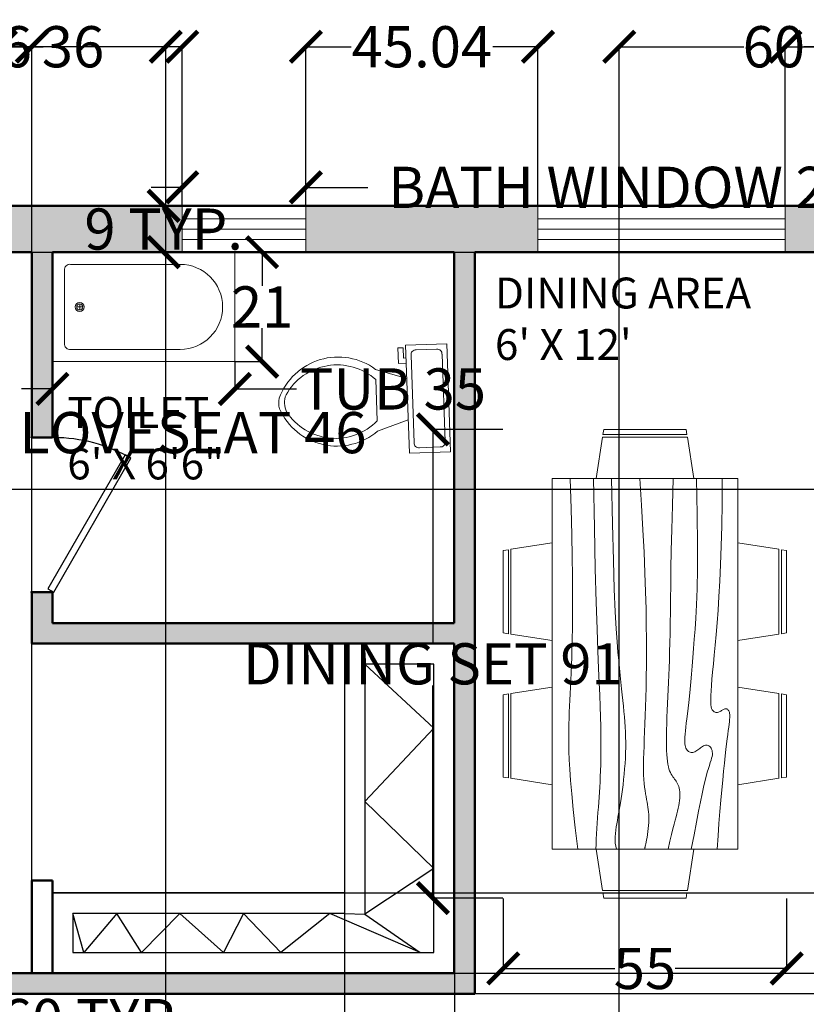
# Model space of a CAD drawing. Units: inches. Extents: x -30 to 744, y -375 to 57.
# Tile 5 of 8: x 202 to 355, y -134 to 57. Entities that reach past the tile are written whole.
import ezdxf

# ---------------------------------------------------------------- set-up
doc = ezdxf.new("R2010")
doc.units = ezdxf.units.IN
doc.header["$MEASUREMENT"] = 0
for name, color, linetype, lineweight in [('A-ANNO-DIMS', 2, 'Continuous', 18), ('A-AREA-IDEN', 7, 'Continuous', 25), ('A-DOOR', 3, 'Continuous', 25), ('A-FLOR-CASE', 8, 'Continuous', 25), ('A-FLOR-FIXT', 9, 'Continuous', 20), ('A-FURN', 8, 'Continuous', 18), ('A-GLAZ', 4, 'Continuous', 18), ('A-WALL', 7, 'Continuous', 50)]:
    doc.layers.add(name, color=color, linetype=linetype, lineweight=lineweight)
doc.layers.add('A-WALL-PATT', color=251, linetype='Continuous', lineweight=13, true_color=0x636466)
doc.styles.get("Standard").update_dxf_attribs({"font": 'arial.ttf'})
doc.dimstyles.get("Standard").update_dxf_attribs({"dimtxt": 8, "dimasz": 6, "dimexe": 0.18, "dimexo": 0.0625, "dimgap": 0.09, "dimtad": 0, "dimtih": 1, "dimtoh": 1, "dimdec": 0, "dimzin": 0, "dimdsep": 46, "dimlunit": 4, "dimtxsty": 'Standard', "dimblk": 'ARCHTICK', "dimcen": 0.09, "dimadec": 0, "dimazin": 0, "dimtfac": 1, "dimtdec": 0, "dimtofl": 0, "dimtmove": 0, "dimatfit": 1, "dimldrblk": 'ARCHTICK', "dimfxl": 1, "dimtolj": 1, "dimtzin": 0, "dimarcsym": 0})

# ---------------------------------------------------------------- blocks, each defined once
blk = doc.blocks.new('*U4')
for p, q in [((0, 0), (0, 6)), ((40, 0), (40, 6))]:
    blk.add_line(p, q)
blk.add_lwpolyline([(0, 0), (34.64, -20), (35.52, -18.48), (0.87, 1.52)], close=True)
blk.add_arc((0, 0), 40, 330, 0)
blk = doc.blocks.new('Dining Set - 36 x 72 in.')
for p, q in [((-22, 27.5), (-22.1562, 26.50042)), ((-22, 27.5), (-6, 27.5)), ((-5.8437, 26.49966), (-6, 27.5)), ((6, 27.5), (5.8438, 26.50042)), ((6, 27.5), (22, 27.5)), ((22.1563, 26.49966), (22, 27.5)), ((-22.2343, 26.00059), (-23.4847, 17.99762)), ((-22.2304, 26), (-5.7608, 26)), ((-5.8416, 26.5), (-22.1534, 26.5)), ((-4.5152, 17.99762), (-5.7655, 25.99926)), ((5.7657, 26.00059), (4.5153, 17.99762)), ((5.7696, 26), (22.2392, 26)), ((22.1584, 26.5), (5.8466, 26.5)), ((23.4848, 17.99762), (22.2345, 25.99926)), ((36, 18), (-36, 18)), ((-36, 18), (-36, -18)), ((36, -18), (36, 18)), ((-45.5, 8), (-44.5004, 8.15617)), ((-45.5, 8), (-45.5, -8)), ((-44.5, -8.15843), (-44.5, 8.15338)), ((-44.0006, 8.23428), (-35.9976, 9.48474)), ((-44, 8.23041), (-44, -8.23915)), ((44.0006, 8.23428), (35.9976, 9.48474)), ((44, 8.23041), (44, -8.23915)), ((44.5, -8.15843), (44.5, 8.15338)), ((45.5, 8), (44.5005, 8.15617)), ((45.5, 8), (45.5, -8)), ((-44.4997, -8.15631), (-45.5, -8)), ((-35.9976, -9.48476), (-43.9993, -8.2345)), ((35.9976, -9.48476), (43.9993, -8.2345)), ((44.4997, -8.15631), (45.5, -8)), ((-36, -18), (36, -18)), ((-22.2343, -26.0006), (-23.4847, -17.99762)), ((-4.5152, -17.99762), (-5.7655, -25.99928)), ((5.7657, -26.0006), (4.5153, -17.99762)), ((23.4848, -17.99762), (22.2345, -25.99928)), ((-22.2304, -26), (-5.7608, -26)), ((-22, -27.5), (-22.1562, -26.50044)), ((-5.8416, -26.5), (-22.1534, -26.5)), ((-5.8437, -26.49967), (-6, -27.5)), ((5.7696, -26), (22.2392, -26)), ((6, -27.5), (5.8438, -26.50044)), ((22.1584, -26.5), (5.8466, -26.5)), ((22.1563, -26.49967), (22, -27.5)), ((-22, -27.5), (-6, -27.5)), ((6, -27.5), (22, -27.5))]:
    blk.add_line(p, q)
for points in [[(-36, 15), (-31.1772, 14.97754), (-26.8079, 14.91406), (-22.8538, 14.81543), (-19.276, 14.6875), (-16.0362, 14.53613), (-13.0957, 14.36718), (-10.4159, 14.18652), (-7.9583, 14), (-5.6904, 13.81315), (-3.6035, 13.63021), (-1.6954, 13.45508), (0.0365, 13.29166), (1.5945, 13.14388), (2.9811, 13.01562), (4.1988, 12.9108), (5.25, 12.83333), (6.1393, 12.78613), (6.8802, 12.76823), (7.4883, 12.77767), (7.9792, 12.8125), (8.3685, 12.87077), (8.6719, 12.95052), (8.9049, 13.0498), (9.0833, 13.16666), (9.2205, 13.29899), (9.3216, 13.44401), (9.3895, 13.59879), (9.4271, 13.76041), (9.4373, 13.92594), (9.4232, 14.09245), (9.3875, 14.257), (9.3333, 14.41666), (9.2638, 14.56917), (9.1836, 14.71484), (9.0975, 14.85465), (9.0104, 14.98958), (8.9272, 15.1206), (8.8529, 15.2487), (8.7922, 15.37483), (8.75, 15.5), (8.7305, 15.62467), (8.7344, 15.74739), (8.7617, 15.86621), (8.8125, 15.97916), (8.8867, 16.08431), (8.9844, 16.17968), (9.1055, 16.26334), (9.25, 16.33333), (9.4189, 16.38802), (9.6172, 16.42708), (9.8506, 16.45052), (10.125, 16.45833), (10.4463, 16.45052), (10.8203, 16.42708), (11.2529, 16.38802), (11.75, 16.33333), (12.3184, 16.26318), (12.9694, 16.17838), (13.7151, 16.07991), (14.5677, 15.96875), (15.5395, 15.84586), (16.6426, 15.71224), (17.8893, 15.56884), (19.2917, 15.41666), (20.859, 15.25667), (22.5879, 15.08984), (24.4721, 14.91715), (26.5052, 14.73958), (28.6809, 14.5581), (30.9929, 14.3737), (33.4347, 14.18733), (36, 14)], [(-36, 10), (-28.9766, 10.14274), (-23.1725, 10.20442), (-18.4241, 10.19775), (-14.5677, 10.13541), (-11.4399, 10.03011), (-8.877, 9.89453), (-6.7154, 9.74137), (-4.7917, 9.58333), (-2.9698, 9.43082), (-1.2246, 9.28515), (0.4415, 9.14534), (2.026, 9.01041), (3.5266, 8.87939), (4.9408, 8.7513), (6.266, 8.62516), (7.5, 8.5), (8.6411, 8.37549), (9.6914, 8.2539), (10.6538, 8.13818), (11.5312, 8.03125), (12.3267, 7.93603), (13.043, 7.85547), (13.6831, 7.79248), (14.25, 7.75), (14.7471, 7.7303), (15.1797, 7.73307), (15.5537, 7.75732), (15.875, 7.80208), (16.1494, 7.86637), (16.3828, 7.94922), (16.5811, 8.04964), (16.75, 8.16666), (16.8944, 8.29915), (17.0143, 8.44531), (17.1089, 8.60319), (17.1771, 8.77083), (17.218, 8.94629), (17.2305, 9.1276), (17.2137, 9.31282), (17.1667, 9.5), (17.0895, 9.6875), (16.987, 9.875), (16.8649, 10.0625), (16.7292, 10.25), (16.5856, 10.4375), (16.4401, 10.625), (16.2985, 10.8125), (16.1667, 11), (16.05, 11.18733), (15.9518, 11.3737), (15.8752, 11.5581), (15.8229, 11.73958), (15.798, 11.91715), (15.8034, 12.08984), (15.842, 12.25667), (15.9167, 12.41666), (16.0295, 12.56836), (16.1784, 12.70833), (16.3605, 12.83268), (16.5729, 12.9375), (16.8127, 13.01888), (17.0768, 13.07291), (17.3625, 13.0957), (17.6667, 13.08333), (17.9894, 13.03312), (18.3418, 12.94726), (18.7382, 12.82918), (19.1927, 12.68229), (19.7195, 12.51001), (20.3327, 12.31575), (21.0465, 12.10294), (21.875, 11.875), (22.8357, 11.63354), (23.959, 11.37304), (25.2786, 11.08618), (26.8282, 10.76562), (28.6414, 10.40405), (30.752, 9.99414), (33.1936, 9.52856), (36, 9)], [(-36, 5.5), (-30.7157, 5.3348), (-26.069, 5.20963), (-21.9946, 5.11767), (-18.4271, 5.05208), (-15.3009, 5.00602), (-12.5508, 4.97265), (-10.1112, 4.94515), (-7.9167, 4.91666), (-5.909, 4.88167), (-4.0586, 4.83984), (-2.3429, 4.79215), (-0.7396, 4.73958), (0.7739, 4.6831), (2.22, 4.6237), (3.6213, 4.56233), (5, 4.5), (6.373, 4.43782), (7.7344, 4.3776), (9.0723, 4.32129), (10.375, 4.27083), (11.6309, 4.22819), (12.8281, 4.19531), (13.9551, 4.17415), (15, 4.16666), (15.954, 4.17448), (16.819, 4.19791), (17.6001, 4.23698), (18.3021, 4.29166), (18.9299, 4.36198), (19.4883, 4.44791), (19.9823, 4.54948), (20.4167, 4.66666), (20.7969, 4.79899), (21.1302, 4.94401), (21.4245, 5.09879), (21.6875, 5.26041), (21.9271, 5.42594), (22.1511, 5.59245), (22.3672, 5.757), (22.5834, 5.91666), (22.8065, 6.06868), (23.0404, 6.21093), (23.2879, 6.34147), (23.5521, 6.45833), (23.8358, 6.55957), (24.142, 6.64323), (24.4735, 6.70735), (24.8334, 6.75), (25.2235, 6.76969), (25.642, 6.76692), (26.0858, 6.74267), (26.5521, 6.69791), (27.0379, 6.63362), (27.5404, 6.55078), (28.0565, 6.45036), (28.5834, 6.33333), (29.1242, 6.19987), (29.7071, 6.04687), (30.3661, 5.87044), (31.1354, 5.66666), (32.0493, 5.43164), (33.142, 5.16146), (34.4475, 4.85221), (36, 4.5)], [(-36, -1), (-30.7915, -0.6591), (-26.0195, -0.38216), (-21.6519, -0.16284), (-17.6563, 0.00521), (-14.0005, 0.12833), (-10.6523, 0.21289), (-7.5796, 0.26522), (-4.75, 0.29166), (-2.134, 0.29793), (0.2878, 0.28711), (2.5317, 0.26163), (4.6146, 0.22396), (6.5529, 0.17651), (8.3633, 0.12174), (10.0623, 0.06209), (11.6667, 0), (13.1899, -0.06201), (14.6341, -0.1211), (15.9982, -0.17432), (17.2813, -0.21875), (18.4823, -0.25147), (19.6003, -0.26953), (20.6343, -0.27002), (21.5834, -0.25), (22.4481, -0.20768), (23.2357, -0.14584), (23.9549, -0.06836), (24.6146, 0.02083), (25.2235, 0.11784), (25.7904, 0.21875), (26.3241, 0.31966), (26.8334, 0.41666), (27.3265, 0.50618), (27.8099, 0.58593), (28.2894, 0.65397), (28.7709, 0.70833), (29.2601, 0.74707), (29.763, 0.76823), (30.2855, 0.76985), (30.8334, 0.75), (31.4088, 0.70784), (31.9994, 0.64713), (32.589, 0.57275), (33.1615, 0.48958), (33.7008, 0.4025), (34.1908, 0.3164), (34.6153, 0.23616), (34.9584, 0.16666), (35.2099, 0.11165), (35.3848, 0.07031), (35.504, 0.04069), (35.5886, 0.02083), (35.6594, 0.00879), (35.7377, 0.0026), (35.8442, 0.00032), (36, 0)], [(-36, -6.5), (-27.1843, -6.31267), (-20.084, -6.1263), (-14.469, -5.9419), (-10.1094, -5.76042), (-6.7752, -5.58285), (-4.2363, -5.41016), (-2.2629, -5.24333), (-0.625, -5.08334), (0.8708, -4.93099), (2.2715, -4.78646), (3.5872, -4.64974), (4.8281, -4.52084), (6.0046, -4.39974), (7.127, -4.28646), (8.2053, -4.18099), (9.25, -4.08334), (10.2705, -3.99382), (11.2734, -3.91407), (12.2647, -3.84603), (13.25, -3.79167), (14.2354, -3.75293), (15.2266, -3.73177), (16.2295, -3.73015), (17.25, -3.75), (18.2912, -3.79248), (19.3451, -3.85547), (20.4009, -3.93604), (21.4479, -4.03125), (22.4754, -4.13819), (23.4727, -4.25391), (24.4289, -4.37549), (25.3334, -4.5), (26.1785, -4.62492), (26.9694, -4.74935), (27.7145, -4.87281), (28.4219, -4.99479), (29.1, -5.11483), (29.7572, -5.23242), (30.4016, -5.34709), (31.0417, -5.45834), (31.6837, -5.56437), (32.3262, -5.65821), (32.9658, -5.73153), (33.599, -5.77604), (34.2224, -5.78345), (34.8327, -5.74545), (35.4264, -5.65373), (36, -5.5)], [(-36, -10), (-26.4022, -9.81299), (-18.4675, -9.62891), (-11.9839, -9.45069), (-6.7396, -9.28125), (-2.5226, -9.12354), (0.8789, -8.98047), (3.6769, -8.85498), (6.0833, -8.75), (8.2767, -8.66765), (10.3021, -8.60677), (12.1712, -8.56543), (13.8958, -8.54167), (15.4876, -8.53353), (16.9583, -8.53907), (18.3197, -8.55632), (19.5834, -8.58334), (20.7616, -8.61841), (21.8685, -8.66081), (22.9188, -8.71004), (23.9271, -8.76563), (24.9081, -8.82707), (25.8763, -8.89388), (26.8465, -8.96558), (27.8334, -9.04167), (28.8474, -9.12118), (29.8828, -9.20117), (30.93, -9.27824), (31.9792, -9.34896), (33.0205, -9.40991), (34.0443, -9.45768), (35.0407, -9.48885), (36, -9.5)], [(-36, -14.5), (-30.0881, -14.33513), (-25.0332, -14.21224), (-20.7312, -14.12647), (-17.0781, -14.07292), (-13.97, -14.04671), (-11.3027, -14.04297), (-8.9724, -14.05681), (-6.875, -14.08334), (-4.9224, -14.11833), (-3.0905, -14.16016), (-1.3709, -14.20785), (0.2448, -14.26042), (1.7647, -14.3169), (3.1973, -14.3763), (4.5507, -14.43767), (5.8333, -14.5), (7.0554, -14.5621), (8.235, -14.62175), (9.3922, -14.67652), (10.5469, -14.72396), (11.7192, -14.76164), (12.929, -14.78711), (14.1965, -14.79794), (15.5417, -14.79167), (16.9933, -14.76424), (18.6152, -14.70508), (20.4804, -14.60197), (22.6615, -14.44271), (25.2312, -14.21509), (28.2624, -13.9069), (31.8277, -13.50594), (36, -13)]]:
    blk.add_lwpolyline(points)
blk = doc.blocks.new('Bath Tub - 26 x 60 in.')
for p, q in [((8, -18), (10, -18)), ((9, -17), (9, -19))]:
    blk.add_line(p, q)
blk.add_lwpolyline([(0, -36), (0, 0), (60, 0), (60, -36)], close=True)
for points in [[(4, -30), (4, -6)], [(6, -4), (42, -4)], [(42, -32), (6, -32)]]:
    blk.add_lwpolyline(points)
for radius in [1.5, 1]:
    blk.add_circle((9, -18), radius)
for centre, radius, start, end in [((5.75, -5.75), 1.77, 81.8699, 188.1301), ((42, -18), 14, 270, 90), ((5.75, -30.25), 1.77, 171.8699, 278.1301)]:
    blk.add_arc(centre, radius, start, end)
blk = doc.blocks.new('Toilet - top')
for p, q in [((9.5, -6), (9.5, -2)), ((-10, -8.5), (-8, -8.5)), ((-10, -9.5), (-10, -8.5)), ((-7, -9.5), (-10, -9.5)), ((-8, -8.5), (-8, -8)), ((-7, -8), (-7, -9.5)), ((-4, -8), (-6, -14)), ((4, -8), (6, -14)), ((4, -14), (-4, -14))]:
    blk.add_line(p, q)
blk.add_lwpolyline([(10.5, -8), (10.5, 0), (-10.5, 0), (-10.5, -8)], close=True)
for points in [[(8.5, -1), (-8.5, -1)], [(-9.5, -2), (-9.5, -6)], [(-8.5, -7), (8.5, -7)]]:
    blk.add_lwpolyline(points)
for centre, radius, start, end in [((-8.62, -1.88), 0.884, 81.8699, 188.1301), ((8.62, -1.88), 0.884, 351.8699, 98.1301), ((-8.62, -6.12), 0.884, 171.8699, 278.1301), ((8.62, -6.12), 0.884, 261.8699, 8.1301), ((3.52, -21.58), 12.17, 141.4691, 247.9714), ((4.2, -21.82), 11.33, 136.3677, 238.9468), ((-3.52, -21.58), 12.17, 292.0284, 38.5307), ((-4.2, -21.82), 11.33, 301.053, 43.6321), ((0, -27.88), 4, 245.7318, 294.2682), ((0, -29), 4, 254.8605, 285.1395)]:
    blk.add_arc(centre, radius, start, end)
blk = doc.blocks.new('WIN-48IN')
for p, q in [((0, 0), (0, 48)), ((0, 48), (9, 48)), ((2.5, 48), (2.5, 0)), ((4.5, 48), (4.5, 0)), ((6.5, 48), (6.5, 0)), ((9, 48), (9, 0)), ((9, 48), (9, 0)), ((9, 0), (0, 0))]:
    blk.add_line(p, q)
blk = doc.blocks.new('WIN-24IN')
for p, q in [((0, 0), (0, 9)), ((0, 9), (24, 9)), ((24, 0), (24, 9)), ((24, 6.5), (0, 6.5)), ((24, 4.5), (0, 4.5)), ((24, 2.5), (0, 2.5)), ((24, 0), (0, 0)), ((24, 0), (0, 0))]:
    blk.add_line(p, q)
blk = doc.blocks.new('_ArchTick')
at = {"color": 0, "linetype": 'ByBlock', "const_width": 0.15}
blk.add_lwpolyline([(-0.5, -0.5), (0.5, 0.5)], dxfattribs=at)
blk = doc.blocks.new('*D38')
at = {"layer": 'A-ANNO-DIMS', "color": 0, "lineweight": -2, "transparency": 16777216}
for p, q in [((208.24, -9.6), (208.24, -15.03)), ((243.64, -9.6), (243.64, -15.03)), ((208.24, -14.85), (202.24, -14.85)), ((243.64, -14.85), (255.64, -14.85))]:
    blk.add_line(p, q, dxfattribs=at)
at = {"layer": 'Defpoints', "color": 0, "transparency": 16777216}
for p in [(208.24, -9.54), (243.64, -9.54), (243.64, -14.85)]:
    blk.add_point(p, dxfattribs=at)
at = {"layer": 'A-ANNO-DIMS', "color": 0, "lineweight": -2, "transparency": 16777216, "xscale": 6, "yscale": 6, "zscale": 6}
blk.add_blockref('_ArchTick', (208.24, -14.85), dxfattribs=at)
at = {"layer": 'A-ANNO-DIMS', "color": 0, "lineweight": -2, "transparency": 16777216, "xscale": 6, "yscale": 6, "zscale": 6, "rotation": 180}
blk.add_blockref('_ArchTick', (243.64, -14.85), dxfattribs=at)
at = {"layer": 'A-ANNO-DIMS', "color": 0, "transparency": 16777216, "insert": (274.32, -14.85), "char_height": 8, "attachment_point": 5}
blk.add_mtext('\\A1;TUB 35', dxfattribs=at)
blk = doc.blocks.new('*D39')
at = {"layer": 'A-ANNO-DIMS', "color": 0, "lineweight": -2, "transparency": 16777216}
for p, q in [((243.7, 11.7), (249.13, 11.7)), ((248.95, 11.7), (248.95, 5.19)), ((248.95, -9.54), (248.95, -3.02)), ((243.7, -9.54), (249.13, -9.54))]:
    blk.add_line(p, q, dxfattribs=at)
at = {"layer": 'Defpoints', "color": 0, "transparency": 16777216}
for p in [(243.64, 11.7), (248.95, 11.7), (243.64, -9.54)]:
    blk.add_point(p, dxfattribs=at)
at = {"layer": 'A-ANNO-DIMS', "color": 0, "lineweight": -2, "transparency": 16777216, "xscale": 6, "yscale": 6, "zscale": 6}
for p, rotation in [((248.95, 11.7), 90), ((248.95, -9.54), 270)]:
    blk.add_blockref('_ArchTick', p, dxfattribs=dict(at, rotation=rotation))
at = {"layer": 'A-ANNO-DIMS', "color": 0, "transparency": 16777216, "insert": (248.95, 1.08), "char_height": 8, "attachment_point": 5}
blk.add_mtext('\\A1;21', dxfattribs=at)
blk = doc.blocks.new('*D42')
at = {"layer": 'A-ANNO-DIMS', "color": 0, "lineweight": -2, "transparency": 16777216}
for p, q in [((233.43, 24.3), (227.43, 24.3)), ((233.43, 20.77), (233.43, 24.48)), ((257.43, 20.77), (257.43, 24.48)), ((257.43, 24.3), (269.43, 24.3))]:
    blk.add_line(p, q, dxfattribs=at)
at = {"layer": 'Defpoints', "color": 0, "transparency": 16777216}
for p in [(257.43, 24.3), (233.43, 20.7), (257.43, 20.7)]:
    blk.add_point(p, dxfattribs=at)
at = {"layer": 'A-ANNO-DIMS', "color": 0, "lineweight": -2, "transparency": 16777216, "xscale": 6, "yscale": 6, "zscale": 6}
blk.add_blockref('_ArchTick', (233.43, 24.3), dxfattribs=at)
at = {"layer": 'A-ANNO-DIMS', "color": 0, "lineweight": -2, "transparency": 16777216, "xscale": 6, "yscale": 6, "zscale": 6, "rotation": 180}
blk.add_blockref('_ArchTick', (257.43, 24.3), dxfattribs=at)
at = {"layer": 'A-ANNO-DIMS', "color": 0, "transparency": 16777216, "insert": (331.34, 24.3), "char_height": 8, "attachment_point": 5}
blk.add_mtext('\\A1;BATH WINDOW 24 TYP.', dxfattribs=at)
blk = doc.blocks.new('*D43')
at = {"layer": 'A-ANNO-DIMS', "color": 0, "lineweight": -2, "transparency": 16777216}
for p, q in [((233.37, 20.7), (229.65, 20.7)), ((229.83, 20.7), (229.83, 20.38)), ((233.37, 11.7), (229.65, 11.7)), ((229.83, 11.7), (229.83, 12.03))]:
    blk.add_line(p, q, dxfattribs=at)
at = {"layer": 'Defpoints', "color": 0, "transparency": 16777216}
for p in [(229.83, 20.7), (233.43, 20.7), (233.43, 11.7)]:
    blk.add_point(p, dxfattribs=at)
at = {"layer": 'A-ANNO-DIMS', "color": 0, "lineweight": -2, "transparency": 16777216, "xscale": 6, "yscale": 6, "zscale": 6}
for p, rotation in [((229.83, 20.7), 90), ((229.83, 11.7), 270)]:
    blk.add_blockref('_ArchTick', p, dxfattribs=dict(at, rotation=rotation))
at = {"layer": 'A-ANNO-DIMS', "color": 0, "transparency": 16777216, "insert": (229.83, 16.2), "char_height": 8, "attachment_point": 5}
blk.add_mtext('\\A1;9 TYP.', dxfattribs=at)
blk = doc.blocks.new('*D44')
at = {"layer": 'A-ANNO-DIMS', "color": 0, "lineweight": -2, "transparency": 16777216}
for p, q in [((53.6, -128.37), (53.6, -137.48)), ((113.6, -128.37), (113.6, -137.48)), ((53.6, -137.3), (47.6, -137.3)), ((113.6, -137.3), (125.6, -137.3))]:
    blk.add_line(p, q, dxfattribs=at)
at = {"layer": 'Defpoints', "color": 0, "transparency": 16777216}
for p in [(53.6, -128.3), (113.6, -128.3), (113.6, -137.3)]:
    blk.add_point(p, dxfattribs=at)
at = {"layer": 'A-ANNO-DIMS', "color": 0, "lineweight": -2, "transparency": 16777216, "xscale": 6, "yscale": 6, "zscale": 6}
blk.add_blockref('_ArchTick', (53.6, -137.3), dxfattribs=at)
at = {"layer": 'A-ANNO-DIMS', "color": 0, "lineweight": -2, "transparency": 16777216, "xscale": 6, "yscale": 6, "zscale": 6, "rotation": 180}
blk.add_blockref('_ArchTick', (113.6, -137.3), dxfattribs=at)
at = {"layer": 'A-ANNO-DIMS', "color": 0, "transparency": 16777216, "insert": (182.83, -137.3), "char_height": 8, "attachment_point": 5}
blk.add_mtext('\\A1;TV CONSOLE 60 TYP.', dxfattribs=at)
blk = doc.blocks.new('*D46')
at = {"layer": 'A-ANNO-DIMS', "color": 0, "lineweight": -2, "transparency": 16777216}
for p, q in [((295.66, -22.72), (281.9, -22.72)), ((282.08, -22.72), (282.08, -63.99)), ((282.08, -113.72), (282.08, -72.44)), ((295.66, -113.72), (281.9, -113.72))]:
    blk.add_line(p, q, dxfattribs=at)
at = {"layer": 'Defpoints', "color": 0, "transparency": 16777216}
for p in [(295.73, -22.72), (282.08, -113.72), (295.73, -113.72)]:
    blk.add_point(p, dxfattribs=at)
at = {"layer": 'A-ANNO-DIMS', "color": 0, "lineweight": -2, "transparency": 16777216, "xscale": 6, "yscale": 6, "zscale": 6}
for p, rotation in [((282.08, -22.72), 90), ((282.08, -113.72), 270)]:
    blk.add_blockref('_ArchTick', p, dxfattribs=dict(at, rotation=rotation))
at = {"layer": 'A-ANNO-DIMS', "color": 0, "transparency": 16777216, "insert": (282.08, -68.22), "char_height": 8, "attachment_point": 5}
blk.add_mtext('\\A1;DINING SET 91', dxfattribs=at)
blk = doc.blocks.new('*D47')
at = {"layer": 'A-ANNO-DIMS', "color": 0, "lineweight": -2, "transparency": 16777216}
for p, q in [((295.73, -113.78), (295.73, -127.55)), ((350.73, -113.78), (350.73, -127.55)), ((295.73, -127.37), (317.38, -127.37)), ((350.73, -127.37), (329.08, -127.37))]:
    blk.add_line(p, q, dxfattribs=at)
at = {"layer": 'Defpoints', "color": 0, "transparency": 16777216}
for p in [(295.73, -113.72), (350.73, -113.72), (350.73, -127.37)]:
    blk.add_point(p, dxfattribs=at)
at = {"layer": 'A-ANNO-DIMS', "color": 0, "lineweight": -2, "transparency": 16777216, "xscale": 6, "yscale": 6, "zscale": 6, "rotation": 180}
blk.add_blockref('_ArchTick', (295.73, -127.37), dxfattribs=at)
at = {"layer": 'A-ANNO-DIMS', "color": 0, "lineweight": -2, "transparency": 16777216, "xscale": 6, "yscale": 6, "zscale": 6}
blk.add_blockref('_ArchTick', (350.73, -127.37), dxfattribs=at)
at = {"layer": 'A-ANNO-DIMS', "color": 0, "transparency": 16777216, "insert": (323.23, -127.37), "char_height": 8, "attachment_point": 5}
blk.add_mtext('\\A1;55', dxfattribs=at)
blk = doc.blocks.new('*D56')
at = {"layer": 'A-ANNO-DIMS', "color": 0, "lineweight": -2, "transparency": 16777216}
for p, q in [((140.35, -16.43), (140.35, -23.51)), ((186.8, -16.43), (186.8, -23.51)), ((140.35, -23.33), (134.35, -23.33)), ((186.8, -23.33), (198.8, -23.33))]:
    blk.add_line(p, q, dxfattribs=at)
at = {"layer": 'Defpoints', "color": 0, "transparency": 16777216}
for p in [(140.35, -16.36), (186.8, -16.36), (186.8, -23.33)]:
    blk.add_point(p, dxfattribs=at)
at = {"layer": 'A-ANNO-DIMS', "color": 0, "lineweight": -2, "transparency": 16777216, "xscale": 6, "yscale": 6, "zscale": 6}
blk.add_blockref('_ArchTick', (140.35, -23.33), dxfattribs=at)
at = {"layer": 'A-ANNO-DIMS', "color": 0, "lineweight": -2, "transparency": 16777216, "xscale": 6, "yscale": 6, "zscale": 6, "rotation": 180}
blk.add_blockref('_ArchTick', (186.8, -23.33), dxfattribs=at)
at = {"layer": 'A-ANNO-DIMS', "color": 0, "transparency": 16777216, "insert": (235.5, -23.33), "char_height": 8, "attachment_point": 5}
blk.add_mtext('\\A1;LOVESEAT 46', dxfattribs=at)
blk = doc.blocks.new('*D63')
at = {"layer": 'A-ANNO-DIMS', "color": 0, "lineweight": -2, "transparency": 16777216}
for p, q in [((542.17, -132.3), (-16.61, -132.3)), ((-16.43, -132.3), (-16.43, -157.12)), ((-16.43, -190.3), (-16.43, -165.47)), ((542.17, -190.3), (-16.61, -190.3))]:
    blk.add_line(p, q, dxfattribs=at)
at = {"layer": 'Defpoints', "color": 0, "transparency": 16777216}
for p in [(-16.43, -132.3), (542.24, -132.3), (542.24, -190.3)]:
    blk.add_point(p, dxfattribs=at)
at = {"layer": 'A-ANNO-DIMS', "color": 0, "lineweight": -2, "transparency": 16777216, "xscale": 6, "yscale": 6, "zscale": 6}
for p, rotation in [((-16.43, -132.3), 90), ((-16.43, -190.3), 270)]:
    blk.add_blockref('_ArchTick', p, dxfattribs=dict(at, rotation=rotation))
at = {"layer": 'A-ANNO-DIMS', "color": 0, "transparency": 16777216, "insert": (-16.43, -161.3), "char_height": 8, "attachment_point": 5}
blk.add_mtext('\\A1;58', dxfattribs=at)
blk = doc.blocks.new('*D69')
at = {"layer": 'A-ANNO-DIMS', "color": 0, "lineweight": -2, "transparency": 16777216}
for p, q in [((31.24, 20.77), (31.24, 51.78)), ((233.43, 20.77), (233.43, 51.78)), ((31.24, 51.6), (118.72, 51.6)), ((233.43, 51.6), (145.95, 51.6))]:
    blk.add_line(p, q, dxfattribs=at)
at = {"layer": 'Defpoints', "color": 0, "transparency": 16777216}
for p in [(233.43, 51.6), (31.24, 20.7), (233.43, 20.7)]:
    blk.add_point(p, dxfattribs=at)
at = {"layer": 'A-ANNO-DIMS', "color": 0, "lineweight": -2, "transparency": 16777216, "xscale": 6, "yscale": 6, "zscale": 6, "rotation": 180}
blk.add_blockref('_ArchTick', (31.24, 51.6), dxfattribs=at)
at = {"layer": 'A-ANNO-DIMS', "color": 0, "lineweight": -2, "transparency": 16777216, "xscale": 6, "yscale": 6, "zscale": 6}
blk.add_blockref('_ArchTick', (233.43, 51.6), dxfattribs=at)
at = {"layer": 'A-ANNO-DIMS', "color": 0, "transparency": 16777216, "insert": (132.33, 51.6), "char_height": 8, "attachment_point": 5}
blk.add_mtext('\\A1;202.2', dxfattribs=at)
blk = doc.blocks.new('*D70')
at = {"layer": 'A-ANNO-DIMS', "color": 0, "lineweight": -2, "transparency": 16777216}
for p, q in [((257.43, 20.77), (257.43, 51.78)), ((302.47, 20.77), (302.47, 51.78)), ((257.43, 51.6), (266.22, 51.6)), ((302.47, 51.6), (293.68, 51.6))]:
    blk.add_line(p, q, dxfattribs=at)
at = {"layer": 'Defpoints', "color": 0, "transparency": 16777216}
for p in [(302.47, 51.6), (257.43, 20.7), (302.47, 20.7)]:
    blk.add_point(p, dxfattribs=at)
at = {"layer": 'A-ANNO-DIMS', "color": 0, "lineweight": -2, "transparency": 16777216, "xscale": 6, "yscale": 6, "zscale": 6, "rotation": 180}
blk.add_blockref('_ArchTick', (257.43, 51.6), dxfattribs=at)
at = {"layer": 'A-ANNO-DIMS', "color": 0, "lineweight": -2, "transparency": 16777216, "xscale": 6, "yscale": 6, "zscale": 6}
blk.add_blockref('_ArchTick', (302.47, 51.6), dxfattribs=at)
at = {"layer": 'A-ANNO-DIMS', "color": 0, "transparency": 16777216, "insert": (279.95, 51.6), "char_height": 8, "attachment_point": 5}
blk.add_mtext('\\A1;45.04', dxfattribs=at)
blk = doc.blocks.new('*D71')
at = {"layer": 'A-ANNO-DIMS', "color": 0, "lineweight": -2, "transparency": 16777216}
for p, q in [((350.47, 20.77), (350.47, 51.78)), ((405.51, 20.77), (405.51, 51.78)), ((350.47, 51.6), (364.37, 51.6)), ((405.51, 51.6), (391.61, 51.6))]:
    blk.add_line(p, q, dxfattribs=at)
at = {"layer": 'Defpoints', "color": 0, "transparency": 16777216}
for p in [(405.51, 51.6), (350.47, 20.7), (405.51, 20.7)]:
    blk.add_point(p, dxfattribs=at)
at = {"layer": 'A-ANNO-DIMS', "color": 0, "lineweight": -2, "transparency": 16777216, "xscale": 6, "yscale": 6, "zscale": 6, "rotation": 180}
blk.add_blockref('_ArchTick', (350.47, 51.6), dxfattribs=at)
at = {"layer": 'A-ANNO-DIMS', "color": 0, "lineweight": -2, "transparency": 16777216, "xscale": 6, "yscale": 6, "zscale": 6}
blk.add_blockref('_ArchTick', (405.51, 51.6), dxfattribs=at)
at = {"layer": 'A-ANNO-DIMS', "color": 0, "transparency": 16777216, "insert": (377.99, 51.6), "char_height": 8, "attachment_point": 5}
blk.add_mtext('\\A1;55.05', dxfattribs=at)
blk = doc.blocks.new('*D73')
at = {"layer": 'A-ANNO-DIMS', "color": 0, "lineweight": -2, "transparency": 16777216}
for p, q in [((194.24, -330.23), (194.24, 51.78)), ((230.24, -330.23), (230.24, 51.78)), ((194.24, 51.6), (206.42, 51.6)), ((230.24, 51.6), (218.05, 51.6))]:
    blk.add_line(p, q, dxfattribs=at)
at = {"layer": 'Defpoints', "color": 0, "transparency": 16777216}
for p in [(230.24, 51.6), (194.24, -330.3), (230.24, -330.3)]:
    blk.add_point(p, dxfattribs=at)
at = {"layer": 'A-ANNO-DIMS', "color": 0, "lineweight": -2, "transparency": 16777216, "xscale": 6, "yscale": 6, "zscale": 6, "rotation": 180}
blk.add_blockref('_ArchTick', (194.24, 51.6), dxfattribs=at)
at = {"layer": 'A-ANNO-DIMS', "color": 0, "lineweight": -2, "transparency": 16777216, "xscale": 6, "yscale": 6, "zscale": 6}
blk.add_blockref('_ArchTick', (230.24, 51.6), dxfattribs=at)
at = {"layer": 'A-ANNO-DIMS', "color": 0, "transparency": 16777216, "insert": (212.24, 51.6), "char_height": 8, "attachment_point": 5}
blk.add_mtext('\\A1;36', dxfattribs=at)
blk = doc.blocks.new('*D74')
at = {"layer": 'A-ANNO-DIMS', "color": 0, "lineweight": -2, "transparency": 16777216}
for p, q in [((318.24, -330.23), (318.24, 51.78)), ((378.24, -330.23), (378.24, 51.78)), ((318.24, 51.6), (342.41, 51.6)), ((378.24, 51.6), (354.06, 51.6))]:
    blk.add_line(p, q, dxfattribs=at)
at = {"layer": 'Defpoints', "color": 0, "transparency": 16777216}
for p in [(378.24, 51.6), (318.24, -330.3), (378.24, -330.3)]:
    blk.add_point(p, dxfattribs=at)
at = {"layer": 'A-ANNO-DIMS', "color": 0, "lineweight": -2, "transparency": 16777216, "xscale": 6, "yscale": 6, "zscale": 6, "rotation": 180}
blk.add_blockref('_ArchTick', (318.24, 51.6), dxfattribs=at)
at = {"layer": 'A-ANNO-DIMS', "color": 0, "lineweight": -2, "transparency": 16777216, "xscale": 6, "yscale": 6, "zscale": 6}
blk.add_blockref('_ArchTick', (378.24, 51.6), dxfattribs=at)
at = {"layer": 'A-ANNO-DIMS', "color": 0, "transparency": 16777216, "insert": (348.24, 51.6), "char_height": 8, "attachment_point": 5}
blk.add_mtext('\\A1;60', dxfattribs=at)
blk = doc.blocks.new('*D75')
at = {"layer": 'A-ANNO-DIMS', "color": 0, "lineweight": -2, "transparency": 16777216}
for p, q in [((40.3, 11.7), (662.32, 11.7)), ((662.14, 11.7), (662.14, -7.12)), ((662.14, -34.3), (662.14, -15.47)), ((40.3, -34.3), (662.32, -34.3))]:
    blk.add_line(p, q, dxfattribs=at)
at = {"layer": 'Defpoints', "color": 0, "transparency": 16777216}
for p in [(40.24, 11.7), (662.14, 11.7), (40.24, -34.3)]:
    blk.add_point(p, dxfattribs=at)
at = {"layer": 'A-ANNO-DIMS', "color": 0, "lineweight": -2, "transparency": 16777216, "xscale": 6, "yscale": 6, "zscale": 6}
for p, rotation in [((662.14, 11.7), 90), ((662.14, -34.3), 270)]:
    blk.add_blockref('_ArchTick', p, dxfattribs=dict(at, rotation=rotation))
at = {"layer": 'A-ANNO-DIMS', "color": 0, "transparency": 16777216, "insert": (662.14, -11.3), "char_height": 8, "attachment_point": 5}
blk.add_mtext('\\A1;46', dxfattribs=at)
blk = doc.blocks.new('*D86')
at = {"layer": 'A-ANNO-DIMS', "color": 0, "lineweight": -2, "transparency": 16777216}
for p, q in [((198.24, -128.23), (198.24, 51.78)), ((204.24, -128.23), (204.24, 51.78)), ((198.24, 51.6), (198.5, 51.6)), ((204.24, 51.6), (203.97, 51.6))]:
    blk.add_line(p, q, dxfattribs=at)
at = {"layer": 'Defpoints', "color": 0, "transparency": 16777216}
for p in [(204.24, 51.6), (198.24, -128.3), (204.24, -128.3)]:
    blk.add_point(p, dxfattribs=at)
at = {"layer": 'A-ANNO-DIMS', "color": 0, "lineweight": -2, "transparency": 16777216, "xscale": 6, "yscale": 6, "zscale": 6, "rotation": 180}
blk.add_blockref('_ArchTick', (198.24, 51.6), dxfattribs=at)
at = {"layer": 'A-ANNO-DIMS', "color": 0, "lineweight": -2, "transparency": 16777216, "xscale": 6, "yscale": 6, "zscale": 6}
blk.add_blockref('_ArchTick', (204.24, 51.6), dxfattribs=at)
at = {"layer": 'A-ANNO-DIMS', "color": 0, "transparency": 16777216, "insert": (201.24, 51.6), "char_height": 8, "attachment_point": 5}
blk.add_mtext('\\A1;6', dxfattribs=at)
blk = doc.blocks.new('*D89')
at = {"layer": 'A-ANNO-DIMS', "color": 0, "lineweight": -2, "transparency": 16777216}
for p, q in [((264.9, -64.36), (264.9, -370.38)), ((286.24, -64.36), (286.24, -370.38)), ((264.9, -370.2), (258.9, -370.2)), ((286.24, -370.2), (298.24, -370.2))]:
    blk.add_line(p, q, dxfattribs=at)
at = {"layer": 'Defpoints', "color": 0, "transparency": 16777216}
for p in [(264.9, -64.3), (286.24, -64.3), (286.24, -370.2)]:
    blk.add_point(p, dxfattribs=at)
at = {"layer": 'A-ANNO-DIMS', "color": 0, "lineweight": -2, "transparency": 16777216, "xscale": 6, "yscale": 6, "zscale": 6}
blk.add_blockref('_ArchTick', (264.9, -370.2), dxfattribs=at)
at = {"layer": 'A-ANNO-DIMS', "color": 0, "lineweight": -2, "transparency": 16777216, "xscale": 6, "yscale": 6, "zscale": 6, "rotation": 180}
blk.add_blockref('_ArchTick', (286.24, -370.2), dxfattribs=at)
at = {"layer": 'A-ANNO-DIMS', "color": 0, "transparency": 16777216, "insert": (311.88, -370.2), "char_height": 8, "attachment_point": 5}
blk.add_mtext('\\A1;21.34', dxfattribs=at)
blk = doc.blocks.new('*D90')
at = {"layer": 'A-ANNO-DIMS', "color": 0, "lineweight": -2, "transparency": 16777216}
for p, q in [((208.3, -112.68), (662.32, -112.68)), ((662.14, -112.68), (662.14, -116.31)), ((662.14, -128.3), (662.14, -124.66)), ((208.3, -128.3), (662.32, -128.3))]:
    blk.add_line(p, q, dxfattribs=at)
at = {"layer": 'Defpoints', "color": 0, "transparency": 16777216}
for p in [(208.24, -112.68), (208.24, -128.3), (662.14, -128.3)]:
    blk.add_point(p, dxfattribs=at)
at = {"layer": 'A-ANNO-DIMS', "color": 0, "lineweight": -2, "transparency": 16777216, "xscale": 6, "yscale": 6, "zscale": 6}
for p, rotation in [((662.14, -112.68), 90), ((662.14, -128.3), 270)]:
    blk.add_blockref('_ArchTick', p, dxfattribs=dict(at, rotation=rotation))
at = {"layer": 'A-ANNO-DIMS', "color": 0, "transparency": 16777216, "insert": (662.14, -120.49), "char_height": 8, "attachment_point": 5}
blk.add_mtext('\\A1;15.617', dxfattribs=at)

msp = doc.modelspace()

# ---------------------------------------------------------------- hatches: boundary and pattern name
at = {"layer": 'A-WALL-PATT'}
h = msp.add_hatch(color=256, dxfattribs=at)
h.dxf.hatch_style = 1
h.paths.add_polyline_path([(40.2356, 11.7031), (204.2356, 11.7031), (204.2356, -24.2969), (208.2356, -24.2969), (208.2356, 11.7031), (233.4275, 11.7031), (233.4275, 20.7031), (31.2356, 20.7031), (31.2356, -34.2969), (40.2356, -34.2969)])
h.paths.add_polyline_path([(40.2356, -82.2969), (31.2356, -82.2969), (31.2356, -132.2969), (40.2356, -132.2969), (51.0767, -132.2969), (111.3137, -132.2969), (111.3137, -143.2969), (120.3137, -143.2969), (120.3137, -132.2969), (156.2356, -132.2969), (156.2356, -128.2969), (113.6001, -128.2969), (113.6001, -128.3034), (53.6001, -128.3034), (40.2356, -128.2969)])
h.paths.add_polyline_path([(302.4681, 20.7031), (257.4275, 20.7031), (257.4275, 11.7031), (286.2356, 11.7031), (286.2356, -60.2969), (208.2356, -60.2969), (208.2356, -54.2969), (204.2356, -54.2969), (204.2356, -64.2969), (208.2356, -64.2969), (286.2356, -64.2969), (286.2356, -128.2969), (264.8954, -128.2969), (208.2356, -128.2969), (204.2356, -128.2969), (198.2356, -128.2969), (198.2356, -132.2969), (290.2356, -132.2969), (290.2356, -128.2969), (290.2356, 11.7031), (302.4681, 11.7031)])
h.paths.add_polyline_path([(405.515, 20.7031), (350.4681, 20.7031), (350.4681, 11.7031), (362.2356, 11.7031), (362.2356, -34.2969), (366.2356, -34.2969), (366.2356, 11.7031), (405.515, 11.7031)])
h.paths.add_polyline_path([(530.2713, 20.7031), (453.515, 20.7031), (453.515, 11.7031), (486.2356, 11.7031), (486.2356, -128.2969), (448.2356, -128.2969), (448.2356, -132.2969), (486.2356, -132.2969), (490.2356, -132.2969), (496.2356, -132.2969), (496.2356, -128.2969), (490.2356, -128.2969), (490.2356, 11.7031), (530.2713, 11.7031)])
h.paths.add_polyline_path([(631.2356, 20.7031), (578.2713, 20.7031), (578.2713, 11.7031), (622.2356, 11.7031), (622.2356, -37.4001), (631.2356, -37.4001)])
h.paths.add_polyline_path([(631.2356, -85.4001), (622.2356, -85.4001), (622.2356, -91.4001), (622.2356, -103.4001), (622.2356, -128.2969), (538.2356, -128.2969), (538.2356, -132.2969), (538.2356, -154.2969), (542.2356, -154.2969), (542.2356, -132.2969), (575.1375, -132.2969), (585.6313, -131.9348), (585.6438, -132.2969), (622.2356, -132.2969), (622.2356, -147.2969), (631.2356, -147.2969)])
h.paths.add_polyline_path([(631.2356, -171.2969), (622.2356, -171.2969), (622.2356, -185.4028), (622.2356, -186.2969), (622.2356, -190.2969), (542.2356, -190.2969), (542.2356, -184.2969), (538.2356, -184.2969), (538.2356, -190.2969), (538.2356, -194.2969), (622.2356, -194.2969), (622.2356, -237.4632), (631.2356, -237.4632)])
h.paths.add_polyline_path([(631.2356, -285.4632), (622.2356, -285.4632), (622.2356, -330.2969), (490.2356, -330.2969), (490.2356, -194.2969), (494.2356, -194.2969), (495.2356, -194.2969), (495.2356, -190.2969), (494.2356, -190.2969), (490.2356, -190.2969), (486.2356, -190.2969), (366.2356, -190.2969), (366.2356, -194.2969), (486.2356, -194.2969), (486.2356, -330.2969), (426.2356, -330.2969), (426.2356, -339.2969), (631.2356, -339.2969)])
h.paths.add_polyline_path([(378.2356, -330.2969), (318.2356, -330.2969), (318.2356, -194.2969), (324.2356, -194.2969), (324.2356, -190.2969), (318.2356, -190.2969), (314.2356, -190.2969), (314.2356, -194.2969), (314.2356, -330.2969), (278.2356, -330.2969), (278.2356, -339.2969), (378.2356, -339.2969)])
h.paths.add_polyline_path([(190.2356, -330.2969), (40.2356, -330.2969), (40.2356, -318.2969), (31.2356, -318.2969), (31.2356, -330.2969), (31.2356, -339.2969), (190.2356, -339.2969)])
h.paths.add_polyline_path([(230.2356, -330.2969), (194.2356, -330.2969), (194.2356, -194.2969), (194.2356, -190.2969), (190.2356, -190.2969), (184.2356, -190.2969), (184.2356, -194.2969), (190.2356, -194.2969), (190.2356, -339.2969), (230.2356, -339.2969)])
h.paths.add_polyline_path([(142.2356, -190.2969), (120.3137, -190.2969), (120.3137, -184.2969), (116.3137, -184.2969), (111.3137, -184.2969), (111.3137, -190.2969), (40.2356, -190.2969), (31.2356, -190.2969), (31.2356, -194.2969), (31.2356, -206.2969), (40.2356, -206.2969), (40.2356, -194.2969), (142.2356, -194.2969)])

# ---------------------------------------------------------------- linework, layer by layer
at = {"layer": 'A-FLOR-CASE'}
for p, q in [((268.8954, -68.2969), (282.2356, -80.73)), ((282.2356, -80.73), (268.8954, -94.9695)), ((268.8954, -94.9695), (282.2356, -107.9707)), ((282.2356, -107.9707), (268.8954, -116.8146)), ((268.8954, -112.6796), (268.8954, -116.8146)), ((214.3436, -124.2969), (212.2356, -116.6796)), ((220.7491, -116.6796), (214.3436, -124.2969)), ((225.5017, -124.2969), (220.7491, -116.6796)), ((232.9405, -116.6796), (225.5017, -124.2969)), ((241.4124, -124.2969), (232.9405, -116.6796)), ((245.3384, -116.6796), (241.4124, -124.2969)), ((252.5706, -124.2969), (245.3384, -116.6796)), ((262.0756, -116.6796), (252.5706, -124.2969)), ((279.6394, -124.2969), (262.0756, -116.6796)), ((264.8954, -116.6796), (268.8954, -116.8146)), ((268.8954, -116.8146), (279.6394, -124.2969))]:
    msp.add_line(p, q, dxfattribs=at)
for points in [[(264.8954, -128.2969), (286.2356, -128.2969), (286.2356, -64.2969), (264.8954, -64.2969), (264.8954, -112.6796)], [(264.8954, -124.2969), (282.2356, -124.2969), (282.2356, -68.2969), (268.8954, -68.2969), (268.8954, -112.6796)], [(264.8954, -112.6796), (208.2356, -112.6796), (208.2356, -128.2969), (286.2356, -128.2969), (286.2356, -112.6796)], [(264.8954, -116.6796), (212.2356, -116.6796), (212.2356, -124.2969), (282.2356, -124.2969), (282.2356, -112.6796)]]:
    msp.add_lwpolyline(points, dxfattribs=at)
at = {"layer": 'A-WALL'}
for p, q in [((40.2356, 11.7031), (204.2356, 11.7031)), ((204.2356, -24.2969), (204.2356, 11.7031)), ((208.2356, 11.7031), (286.2356, 11.7031)), ((208.2356, -24.2969), (208.2356, 11.7031)), ((286.2356, 11.7031), (286.2356, -60.2969)), ((290.2356, 11.7031), (290.2356, -128.2969)), ((290.2356, 11.7031), (362.2356, 11.7031)), ((208.2356, -24.2969), (204.2356, -24.2969)), ((208.2356, -54.2969), (204.2356, -54.2969)), ((204.2356, -64.2969), (204.2356, -54.2969)), ((208.2356, -60.2969), (208.2356, -54.2969)), ((208.2356, -60.2969), (286.2356, -60.2969)), ((208.2356, -64.2969), (204.2356, -64.2969)), ((208.2356, -64.2969), (286.2356, -64.2969)), ((286.2356, -64.2969), (286.2356, -128.2969)), ((204.2356, -128.2969), (204.2356, -110.2969)), ((208.2356, -110.2969), (204.2356, -110.2969)), ((208.2356, -128.2969), (208.2356, -110.2969)), ((198.2356, -128.2969), (204.2356, -128.2969)), ((208.2356, -128.2969), (204.2356, -128.2969)), ((208.2356, -128.2969), (286.2356, -128.2969)), ((290.2356, -128.2969), (290.2356, -132.2969)), ((198.2356, -132.2969), (290.2356, -132.2969))]:
    msp.add_line(p, q, dxfattribs=at)
msp.add_lwpolyline([(31.2356, -132.2969), (31.2356, 20.7031), (631.2356, 20.7031), (631.2356, -339.2969), (190.2356, -339.2969)], dxfattribs=at)

# ---------------------------------------------------------------- block references
at = {"layer": 'A-DOOR', "xscale": 0.75, "yscale": 0.75, "zscale": 0.75, "rotation": 90}
msp.add_blockref('*U4', (208.4856, -54.2969), dxfattribs=at)
at = {"layer": 'A-FLOR-FIXT', "xscale": 0.5900833548780162, "yscale": 0.5900833548780162, "zscale": 0.5900833548780162}
msp.add_blockref('Bath Tub - 26 x 60 in.', (208.2356, 11.7031), dxfattribs=at)
at = {"layer": 'A-FLOR-FIXT', "rotation": 271.9763442397783}
msp.add_blockref('Toilet - top', (285.14, -16.5541), dxfattribs=at)
at = {"layer": 'A-FURN', "rotation": 270.0000000000001}
msp.add_blockref('Dining Set - 36 x 72 in.', (323.2252, -68.218), dxfattribs=at)
at = {"layer": 'A-GLAZ'}
msp.add_blockref('WIN-24IN', (233.428, 11.703), dxfattribs=at)
at = {"layer": 'A-GLAZ', "rotation": 270.0000000000003}
msp.add_blockref('WIN-48IN', (302.4682, 20.7027), dxfattribs=at)

# ---------------------------------------------------------------- texts
at = {"layer": 'A-AREA-IDEN', "char_height": 6, "attachment_point": 1}
for s, width, insert in [("DINING AREA \\P6' X 12'", 68.113099, (294.1225, 6.7786)), ('TOILET\\P6\' X 6\'6"', 50.515222, (211.1335, -16.4096))]:
    msp.add_mtext_dynamic_manual_height_columns(s, width=width, gutter_width=1, heights=[0], dxfattribs=dict(at, insert=insert))

# ---------------------------------------------------------------- dimensions: what is measured, and where the dimension line sits
at = {"layer": 'A-ANNO-DIMS'}
for base, p1, p2, override, picture, middle in [((233.4275, 51.6031), (31.2356, 20.7031), (233.4275, 20.7031), {"dimdec": 1, "dimlfac": 1, "dimrnd": 0, "dimzin": 0, "dimdsep": 46, "dimlunit": 2}, '*D69', (132.3315, 51.6031)), ((230.2356, 51.6031), (194.2356, -330.2969), (230.2356, -330.2969), {"dimdec": 0, "dimlfac": 1, "dimrnd": 0, "dimzin": 0, "dimdsep": 46, "dimlunit": 2}, '*D73', (212.2356, 51.6031)), ((204.2356, 51.6031), (198.2356, -128.2969), (204.2356, -128.2969), {"dimdec": 0, "dimlfac": 1, "dimrnd": 0, "dimzin": 0, "dimdsep": 46, "dimlunit": 2}, '*D86', (201.2356, 51.6031)), ((302.4681, 51.6031), (257.4275, 20.7031), (302.4681, 20.7031), {"dimdec": 2, "dimlfac": 1, "dimrnd": 0, "dimzin": 0, "dimdsep": 46, "dimlunit": 2}, '*D70', (279.9478, 51.6031)), ((378.2356, 51.6031), (318.2356, -330.2969), (378.2356, -330.2969), {"dimdec": 0, "dimlfac": 1, "dimrnd": 0, "dimzin": 0, "dimdsep": 46, "dimlunit": 2}, '*D74', (348.2356, 51.6031)), ((405.515, 51.6031), (350.4681, 20.7031), (405.515, 20.7031), {"dimdec": 2, "dimlfac": 1, "dimrnd": 0, "dimzin": 0, "dimdsep": 46, "dimlunit": 2}, '*D71', (377.9915, 51.6031)), ((286.2356, -370.1969), (264.8954, -64.2969), (286.2356, -64.2969), {"dimdec": 2, "dimlfac": 1, "dimrnd": 0, "dimzin": 0, "dimdsep": 46, "dimlunit": 2}, '*D89', (311.8754, -370.1969))]:
    dim = msp.add_linear_dim(base=base, p1=p1, p2=p2, dimstyle='Standard', override=override, dxfattribs=at)
    dim.commit()
    dim.dimension.update_dxf_attribs({"geometry": picture, "text_midpoint": middle})
for base, p1, p2, text, picture, middle in [((257.4275, 24.3031), (233.4275, 20.7031), (257.4275, 20.7031), 'BATH WINDOW <> TYP.', '*D42', (331.3374, 24.3031)), ((243.6406, -14.8506), (208.2356, -9.5399), (243.6406, -9.5399), 'TUB <>', '*D38', (274.3199, -14.8506)), ((186.8015, -23.333), (140.3453, -16.3645), (186.8015, -16.3645), 'LOVESEAT <>', '*D56', (235.4973, -23.333)), ((113.6001, -137.3034), (53.6001, -128.3034), (113.6001, -128.3034), 'TV CONSOLE <> TYP.', '*D44', (182.8334, -137.3034))]:
    dim = msp.add_linear_dim(base=base, p1=p1, p2=p2, text=text, dimstyle='Standard', override={"dimdec": 0, "dimlfac": 1, "dimrnd": 0, "dimzin": 0, "dimdsep": 46, "dimlunit": 2}, dxfattribs=at)
    dim.commit()
    dim.dimension.update_dxf_attribs({"geometry": picture, "text_midpoint": middle})
for base, p1, p2, angle, text, picture, middle in [((229.8275, 20.7031), (233.4275, 11.7031), (233.4275, 20.7031), 90, '<> TYP.', '*D43', (229.8275, 16.2031)), ((282.0752, -113.718), (295.7252, -22.718), (295.7252, -113.718), 270, 'DINING SET <>', '*D46', (282.0752, -68.218))]:
    dim = msp.add_linear_dim(base=base, p1=p1, p2=p2, angle=angle, text=text, dimstyle='Standard', override={"dimdec": 0, "dimlfac": 1, "dimrnd": 0, "dimzin": 0, "dimdsep": 46, "dimlunit": 2}, dxfattribs=at)
    dim.commit()
    dim.dimension.update_dxf_attribs({"geometry": picture, "text_midpoint": middle})
for base, p1, p2, angle, override, picture, middle in [((662.1356, 11.7031), (40.2356, -34.2969), (40.2356, 11.7031), 90, {"dimdec": 0, "dimlfac": 1, "dimrnd": 0, "dimzin": 0, "dimdsep": 46, "dimlunit": 2}, '*D75', (662.1356, -11.2969)), ((248.9513, 11.7031), (243.6406, -9.5399), (243.6406, 11.7031), 90, {"dimdec": 0, "dimlfac": 1, "dimrnd": 0, "dimzin": 0, "dimdsep": 46, "dimlunit": 2}, '*D39', (248.9513, 1.0816)), ((662.1356, -128.2969), (208.2356, -112.6796), (208.2356, -128.2969), 90, {"dimdec": 3, "dimlfac": 1, "dimrnd": 0, "dimzin": 0, "dimdsep": 46, "dimlunit": 2}, '*D90', (662.1356, -120.4882)), ((350.7252, -127.368), (295.7252, -113.718), (350.7252, -113.718), 0, {"dimdec": 0, "dimlfac": 1, "dimrnd": 0, "dimzin": 0, "dimdsep": 46, "dimlunit": 2}, '*D47', (323.2252, -127.368)), ((-16.4253, -132.2969), (542.2356, -190.2969), (542.2356, -132.2969), 90, {"dimdec": 0, "dimlfac": 1, "dimrnd": 0, "dimzin": 0, "dimdsep": 46, "dimlunit": 2}, '*D63', (-16.4253, -161.2969))]:
    dim = msp.add_linear_dim(base=base, p1=p1, p2=p2, angle=angle, dimstyle='Standard', override=override, dxfattribs=at)
    dim.commit()
    dim.dimension.update_dxf_attribs({"geometry": picture, "text_midpoint": middle})

doc.saveas('drawing.dxf')
